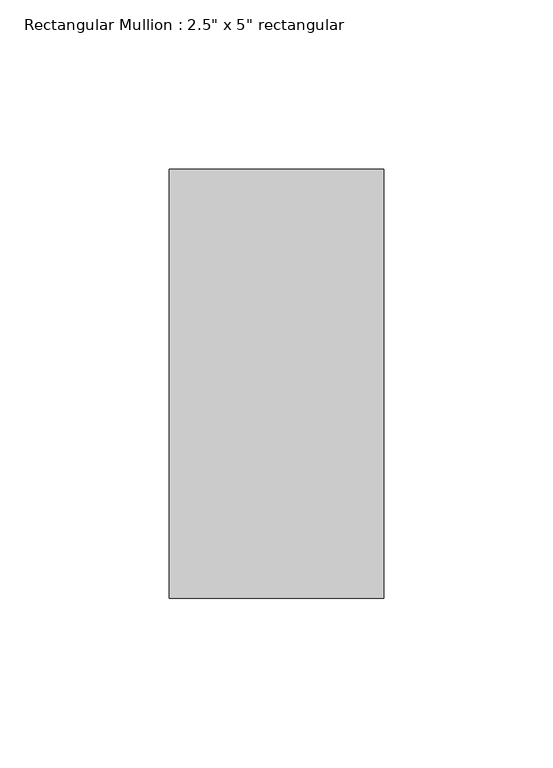
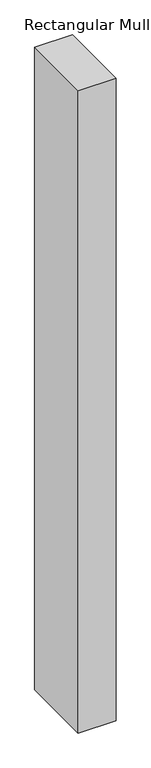
"""IFC4 building model written with IfcOpenShell, lengths in millimetres: member geometry."""

from ifc_helpers import new_model, si_unit, frame, origin, place, context, project, spatial, polyline, outline, extrude, source, transform, mapped, element, save


def member_c84aaad6(model_context):
    return source(origin(), model_context, "Body", "SweptSolid", [
        extrude(outline(polyline([(31.75, 63.5), (31.75, -63.5), (-31.75, -63.5), (-31.75, 63.5), (31.75, 63.5)])), frame((0.0, 0.0, -1142.3751745), z_axis=(0.0, 0.0, 1.0), x_axis=(1.0, 0.0, 0.0)), (0.0, 0.0, 1.0), 1142.3751745),
    ])


if __name__ == "__main__":
    model = new_model("IFC4")
    model_context = context("Model", 3, world=origin())
    ifc_project = project(units=[si_unit("LENGTHUNIT", "METRE", prefix="MILLI")], contexts=[model_context])
    site = spatial("IfcSite", under=ifc_project)
    building = spatial("IfcBuilding", under=site)
    placement = place(None, origin())
    member_shape = member_c84aaad6(model_context)
    element("IfcMember", 1, ObjectType="Rectangular Mullion : 2.5\" x 5\" rectangular", at=placement, inside=building, context=model_context, shape_type="MappedRepresentation", body=[
        mapped(member_shape, transform((0.0, 0.0, 0.0), x_axis=(1.0, 0.0, 0.0), y_axis=(0.0, 1.0, 0.0), z_axis=(0.0, 0.0, 1.0))),
    ])
    save(model, "model.ifc")

# Revit data of these elements
# Type "Rectangular Mullion : 2.5\" x 5\" rectangular"
#   built-in parameter 1007304 = 0.416667 (stored number, unit not read)
#   built-in parameter 1007301 = 0.104167 (stored number, unit not read)
#   built-in parameter 1007300 = 0.104167 (stored number, unit not read)
# Element 1 (IfcMember, "Rectangular Mullion : 2.5\" x 5\" rectangular")
#   Materials on its faces: "Aluminum"
# Materials
#   "Aluminum": class "Metal", colour RGB 247 247 247, transparency 0, Description = "Aluminum 6061", Cost = 0
